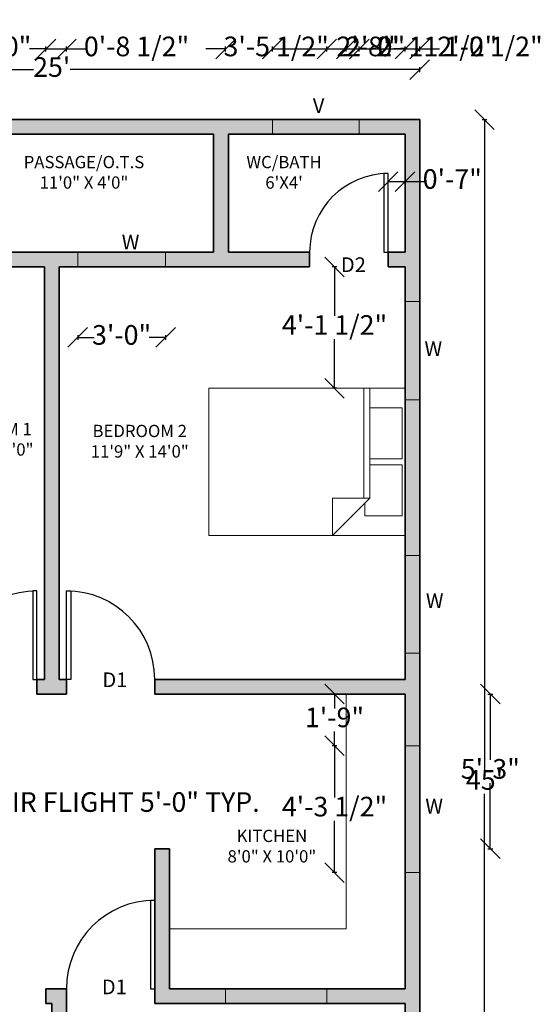
# Model space of a CAD drawing. Units: inches. Extents: x 2247 to 2713, y 588 to 1209.
# Tile 5 of 5: x 2501 to 2713, y 808 to 1209. Entities that reach past the tile are written whole.
import ezdxf

# ---------------------------------------------------------------- set-up
doc = ezdxf.new("R2010")
doc.units = ezdxf.units.IN
for name, color, linetype, lineweight in [('A-ANNO-DIMS', 2, 'Continuous', 18), ('A-ANNO-TEXT', 7, 'Continuous', 18), ('A-AREA-IDEN', 7, 'Continuous', 25), ('A-DOOR', 3, 'Continuous', 25), ('A-FLOR-FIXT', 9, 'Continuous', 18), ('A-FURN', 8, 'Continuous', 18), ('A-GLAZ', 4, 'Continuous', 18), ('A-GLAZ-PATT', 7, 'Continuous', 13), ('A-WALL', 7, 'Continuous', 35), ('A-WALL-PATT', 4, 'Continuous', 13)]:
    doc.layers.add(name, color=color, linetype=linetype, lineweight=lineweight)
doc.styles.get("Standard").update_dxf_attribs({"font": 'arial.ttf'})
doc.dimstyles.new('ISO-25', dxfattribs={"dimtxt": 8, "dimasz": 8, "dimexe": 1, "dimexo": 1, "dimtad": 0, "dimtih": 1, "dimtoh": 1, "dimlunit": 3, "dimtxsty": 'Standard', "dimblk": 'OBLIQUE', "dimcen": 2.5, "dimadec": 0, "dimazin": 0, "dimtfac": 1, "dimtmove": 0, "dimatfit": 3, "dimfxl": 1, "dimfxlon": 1, "dimarcsym": 0})

# ---------------------------------------------------------------- blocks, each defined once
blk = doc.blocks.new('*U4')
for p, q in [((0, 0), (0, -6)), ((-36, 0), (-36, -6))]:
    blk.add_line(p, q)
blk.add_lwpolyline([(0, 0), (0, 36), (-1.75, 36), (-1.75, 0)], close=True)
blk.add_arc((0, 0), 36, 90, 180)
blk = doc.blocks.new('*U6')
for p, q in [((0, 0), (0, -6)), ((-32, 0), (-32, -6))]:
    blk.add_line(p, q)
blk.add_lwpolyline([(0, 0), (0, 32), (-1.75, 32), (-1.75, 0)], close=True)
blk.add_arc((0, 0), 32, 90, 180)
blk = doc.blocks.new('*U5')
for p, q in [((0, 0), (0, -6)), ((36, 0), (36, -6))]:
    blk.add_line(p, q)
blk.add_lwpolyline([(0, 0), (0, 36), (1.75, 36), (1.75, 0)], close=True)
blk.add_arc((0, 0), 36, 0, 90)
blk = doc.blocks.new('Bed - Queen')
for p, q in [((0, -80.00003), (0, 0)), ((0, 0), (59.99999, 0)), ((59.99999, 0), (59.99999, -80.00003)), ((7.99999, -1.2), (28.79998, -1.2)), ((7.99999, -14.4), (7.99999, -1.2)), ((28.79998, -1.2), (28.79998, -14.4)), ((31.19999, -1.2), (51.99999, -1.2)), ((31.19999, -14.4), (31.19999, -1.2)), ((51.99999, -1.2), (51.99999, -16.4)), ((0, -14.4), (44.8, -14.4)), ((59.99999, -29.6), (44.8, -14.4)), ((44.8, -14.4), (44.8, -29.6)), ((44.8, -16.8), (0, -16.8)), ((51.99999, -16.4), (46.79936, -16.4)), ((44.8, -29.6), (59.99999, -29.6)), ((59.99999, -80.00003), (0, -80.00003))]:
    blk.add_line(p, q)
blk = doc.blocks.new('_Oblique')
at = {"color": 0, "linetype": 'ByBlock', "lineweight": -2}
blk.add_line((-0.5, -0.5), (0.5, 0.5), dxfattribs=at)
blk = doc.blocks.new('*D11')
at = {"layer": 'A-ANNO-DIMS', "color": 0, "lineweight": -2, "transparency": 16777216}
for p, q in [((2364.08, 1187.64), (2364.08, 1189.64)), ((2364.08, 1188.64), (2506.59, 1188.64)), ((2664.08, 1188.64), (2521.56, 1188.64)), ((2664.08, 1187.64), (2664.08, 1189.64))]:
    blk.add_line(p, q, dxfattribs=at)
at = {"layer": 'Defpoints', "color": 0, "transparency": 16777216}
for p in [(2664.08, 1188.64), (2364.08, 1168.28), (2664.08, 1168.28)]:
    blk.add_point(p, dxfattribs=at)
at = {"layer": 'A-ANNO-DIMS', "color": 0, "lineweight": -2, "transparency": 16777216, "xscale": 8, "yscale": 8, "zscale": 8, "rotation": 180}
blk.add_blockref('_Oblique', (2364.08, 1188.64), dxfattribs=at)
at = {"layer": 'A-ANNO-DIMS', "color": 0, "lineweight": -2, "transparency": 16777216, "xscale": 8, "yscale": 8, "zscale": 8}
blk.add_blockref('_Oblique', (2664.08, 1188.64), dxfattribs=at)
at = {"layer": 'A-ANNO-DIMS', "color": 0, "transparency": 16777216, "insert": (2514.08, 1188.64), "char_height": 8, "attachment_point": 5}
blk.add_mtext("25'", dxfattribs=at)
blk = doc.blocks.new('*D12')
at = {"layer": 'A-ANNO-DIMS', "color": 0, "lineweight": -2, "transparency": 16777216}
for p, q in [((2689.46, 1168.28), (2691.46, 1168.28)), ((2690.46, 1168.28), (2690.46, 902.97)), ((2690.46, 628.28), (2690.46, 893.59)), ((2689.46, 628.28), (2691.46, 628.28))]:
    blk.add_line(p, q, dxfattribs=at)
at = {"layer": 'Defpoints', "color": 0, "transparency": 16777216}
for p in [(2664.08, 1168.28), (2664.08, 628.28), (2690.46, 628.28)]:
    blk.add_point(p, dxfattribs=at)
at = {"layer": 'A-ANNO-DIMS', "color": 0, "lineweight": -2, "transparency": 16777216, "xscale": 8, "yscale": 8, "zscale": 8}
for p, rotation in [((2690.46, 1168.28), 90), ((2690.46, 628.28), 270)]:
    blk.add_blockref('_Oblique', p, dxfattribs=dict(at, rotation=rotation))
at = {"layer": 'A-ANNO-DIMS', "color": 0, "transparency": 16777216, "insert": (2690.46, 898.28), "char_height": 8, "attachment_point": 5}
blk.add_mtext("45'", dxfattribs=at)
blk = doc.blocks.new('*D17')
at = {"layer": 'A-ANNO-DIMS', "color": 0, "lineweight": -2, "transparency": 16777216}
for p, q in [((2406.08, 890.28), (2406.08, 888.28)), ((2466.08, 890.28), (2466.08, 888.28)), ((2406.08, 889.28), (2466.08, 889.28)), ((2466.08, 889.28), (2474.08, 889.28))]:
    blk.add_line(p, q, dxfattribs=at)
at = {"layer": 'Defpoints', "color": 0, "transparency": 16777216}
for p in [(2406.08, 898.28), (2466.08, 898.28), (2466.08, 889.28)]:
    blk.add_point(p, dxfattribs=at)
at = {"layer": 'A-ANNO-DIMS', "color": 0, "lineweight": -2, "transparency": 16777216, "xscale": 8, "yscale": 8, "zscale": 8, "rotation": 180}
blk.add_blockref('_Oblique', (2406.08, 889.28), dxfattribs=at)
at = {"layer": 'A-ANNO-DIMS', "color": 0, "lineweight": -2, "transparency": 16777216, "xscale": 8, "yscale": 8, "zscale": 8}
blk.add_blockref('_Oblique', (2466.08, 889.28), dxfattribs=at)
at = {"layer": 'A-ANNO-DIMS', "color": 0, "transparency": 16777216, "insert": (2538.49, 889.28), "char_height": 8, "attachment_point": 5}
blk.add_mtext('STAIR FLIGHT 5\'-0" TYP.', dxfattribs=at)
blk = doc.blocks.new('*D26')
at = {"layer": 'A-ANNO-DIMS', "color": 0, "lineweight": -2, "transparency": 16777216}
for p, q in [((2520.08, 600.53), (2520.08, 598.53)), ((2520.08, 599.53), (2526.82, 599.53)), ((2556.08, 599.53), (2549.33, 599.53)), ((2556.08, 600.53), (2556.08, 598.53))]:
    blk.add_line(p, q, dxfattribs=at)
at = {"layer": 'Defpoints', "color": 0, "transparency": 16777216}
for p in [(2520.08, 808.28), (2556.08, 808.28), (2556.08, 599.53)]:
    blk.add_point(p, dxfattribs=at)
at = {"layer": 'A-ANNO-DIMS', "color": 0, "lineweight": -2, "transparency": 16777216, "xscale": 8, "yscale": 8, "zscale": 8, "rotation": 180}
blk.add_blockref('_Oblique', (2520.08, 599.53), dxfattribs=at)
at = {"layer": 'A-ANNO-DIMS', "color": 0, "lineweight": -2, "transparency": 16777216, "xscale": 8, "yscale": 8, "zscale": 8}
blk.add_blockref('_Oblique', (2556.08, 599.53), dxfattribs=at)
at = {"layer": 'A-ANNO-DIMS', "color": 0, "transparency": 16777216, "insert": (2538.08, 599.53), "char_height": 8, "attachment_point": 5}
blk.add_mtext('3\'-0"', dxfattribs=at)
blk = doc.blocks.new('*D38')
at = {"layer": 'A-ANNO-DIMS', "color": 0, "lineweight": -2, "transparency": 16777216}
for p, q in [((2630.33, 913.24), (2628.33, 913.24)), ((2629.33, 913.24), (2629.33, 892.18)), ((2629.33, 861.58), (2629.33, 882.65)), ((2630.33, 861.58), (2628.33, 861.58))]:
    blk.add_line(p, q, dxfattribs=at)
at = {"layer": 'Defpoints', "color": 0, "transparency": 16777216}
for p in [(2629.33, 913.24), (2658.08, 913.24), (2658.08, 861.58)]:
    blk.add_point(p, dxfattribs=at)
at = {"layer": 'A-ANNO-DIMS', "color": 0, "lineweight": -2, "transparency": 16777216, "xscale": 8, "yscale": 8, "zscale": 8}
for p, rotation in [((2629.33, 913.24), 90), ((2629.33, 861.58), 270)]:
    blk.add_blockref('_Oblique', p, dxfattribs=dict(at, rotation=rotation))
at = {"layer": 'A-ANNO-DIMS', "color": 0, "transparency": 16777216, "insert": (2629.33, 887.41), "char_height": 8, "attachment_point": 5}
blk.add_mtext('4\'-3 1/2"', dxfattribs=at)
blk = doc.blocks.new('*D39')
at = {"layer": 'A-ANNO-DIMS', "color": 0, "lineweight": -2, "transparency": 16777216}
for p, q in [((2630.33, 934.28), (2628.33, 934.28)), ((2629.33, 934.28), (2629.33, 928.47)), ((2629.33, 913.24), (2629.33, 919.05)), ((2630.33, 913.24), (2628.33, 913.24))]:
    blk.add_line(p, q, dxfattribs=at)
at = {"layer": 'Defpoints', "color": 0, "transparency": 16777216}
for p in [(2629.33, 934.28), (2658.08, 934.28), (2658.08, 913.24)]:
    blk.add_point(p, dxfattribs=at)
at = {"layer": 'A-ANNO-DIMS', "color": 0, "lineweight": -2, "transparency": 16777216, "xscale": 8, "yscale": 8, "zscale": 8}
for p, rotation in [((2629.33, 934.28), 90), ((2629.33, 913.24), 270)]:
    blk.add_blockref('_Oblique', p, dxfattribs=dict(at, rotation=rotation))
at = {"layer": 'A-ANNO-DIMS', "color": 0, "transparency": 16777216, "insert": (2629.33, 923.76), "char_height": 8, "attachment_point": 5}
blk.add_mtext('1\'-9"', dxfattribs=at)
blk = doc.blocks.new('*D40')
at = {"layer": 'A-ANNO-DIMS', "color": 0, "lineweight": -2, "transparency": 16777216}
for p, q in [((2634.08, 1196.03), (2634.08, 1198.03)), ((2634.08, 1197.03), (2634.75, 1197.03)), ((2658.08, 1197.03), (2657.4, 1197.03)), ((2658.08, 1196.03), (2658.08, 1198.03))]:
    blk.add_line(p, q, dxfattribs=at)
at = {"layer": 'Defpoints', "color": 0, "transparency": 16777216}
for p in [(2658.08, 1197.03), (2634.08, 838.69), (2658.08, 814.28)]:
    blk.add_point(p, dxfattribs=at)
at = {"layer": 'A-ANNO-DIMS', "color": 0, "lineweight": -2, "transparency": 16777216, "xscale": 8, "yscale": 8, "zscale": 8, "rotation": 180}
blk.add_blockref('_Oblique', (2634.08, 1197.03), dxfattribs=at)
at = {"layer": 'A-ANNO-DIMS', "color": 0, "lineweight": -2, "transparency": 16777216, "xscale": 8, "yscale": 8, "zscale": 8}
blk.add_blockref('_Oblique', (2658.08, 1197.03), dxfattribs=at)
at = {"layer": 'A-ANNO-DIMS', "color": 0, "transparency": 16777216, "insert": (2646.08, 1197.03), "char_height": 8, "attachment_point": 5}
blk.add_mtext('2\'-0"', dxfattribs=at)
blk = doc.blocks.new('*D42')
at = {"layer": 'A-ANNO-DIMS', "color": 0, "lineweight": -2, "transparency": 16777216}
for p, q in [((2604.04, 1196.03), (2604.04, 1198.03)), ((2604.04, 1197.03), (2639.39, 1197.03)), ((2639.39, 1196.03), (2639.39, 1198.03)), ((2639.39, 1197.03), (2647.39, 1197.03))]:
    blk.add_line(p, q, dxfattribs=at)
at = {"layer": 'Defpoints', "color": 0, "transparency": 16777216}
for p in [(2639.39, 1197.03), (2604.04, 1168.28), (2639.39, 1168.28)]:
    blk.add_point(p, dxfattribs=at)
at = {"layer": 'A-ANNO-DIMS', "color": 0, "lineweight": -2, "transparency": 16777216, "xscale": 8, "yscale": 8, "zscale": 8, "rotation": 180}
blk.add_blockref('_Oblique', (2604.04, 1197.03), dxfattribs=at)
at = {"layer": 'A-ANNO-DIMS', "color": 0, "lineweight": -2, "transparency": 16777216, "xscale": 8, "yscale": 8, "zscale": 8}
blk.add_blockref('_Oblique', (2639.39, 1197.03), dxfattribs=at)
at = {"layer": 'A-ANNO-DIMS', "color": 0, "transparency": 16777216, "insert": (2671.15, 1197.03), "char_height": 8, "attachment_point": 5}
blk.add_mtext('2\'-11 1/2"', dxfattribs=at)
blk = doc.blocks.new('*D44')
at = {"layer": 'A-ANNO-DIMS', "color": 0, "lineweight": -2, "transparency": 16777216}
for p, q in [((2639.39, 1196.03), (2639.39, 1198.03)), ((2639.39, 1197.03), (2664.08, 1197.03)), ((2664.08, 1196.03), (2664.08, 1198.03)), ((2664.08, 1197.03), (2672.08, 1197.03))]:
    blk.add_line(p, q, dxfattribs=at)
at = {"layer": 'Defpoints', "color": 0, "transparency": 16777216}
for p in [(2664.08, 1197.03), (2639.39, 1168.28), (2664.08, 1168.28)]:
    blk.add_point(p, dxfattribs=at)
at = {"layer": 'A-ANNO-DIMS', "color": 0, "lineweight": -2, "transparency": 16777216, "xscale": 8, "yscale": 8, "zscale": 8, "rotation": 180}
blk.add_blockref('_Oblique', (2639.39, 1197.03), dxfattribs=at)
at = {"layer": 'A-ANNO-DIMS', "color": 0, "lineweight": -2, "transparency": 16777216, "xscale": 8, "yscale": 8, "zscale": 8}
blk.add_blockref('_Oblique', (2664.08, 1197.03), dxfattribs=at)
at = {"layer": 'A-ANNO-DIMS', "color": 0, "transparency": 16777216, "insert": (2692.72, 1197.03), "char_height": 8, "attachment_point": 5}
blk.add_mtext('2\'-0 1/2"', dxfattribs=at)
blk = doc.blocks.new('*D45')
at = {"layer": 'A-ANNO-DIMS', "color": 0, "lineweight": -2, "transparency": 16777216}
for p, q in [((2456.06, 600.53), (2456.06, 598.53)), ((2456.06, 599.53), (2487.37, 599.53)), ((2487.37, 600.53), (2487.37, 598.53)), ((2487.37, 599.53), (2495.37, 599.53))]:
    blk.add_line(p, q, dxfattribs=at)
at = {"layer": 'Defpoints', "color": 0, "transparency": 16777216}
for p in [(2456.06, 1108.28), (2487.37, 1108.28), (2487.37, 599.53)]:
    blk.add_point(p, dxfattribs=at)
at = {"layer": 'A-ANNO-DIMS', "color": 0, "lineweight": -2, "transparency": 16777216, "xscale": 8, "yscale": 8, "zscale": 8, "rotation": 180}
blk.add_blockref('_Oblique', (2456.06, 599.53), dxfattribs=at)
at = {"layer": 'A-ANNO-DIMS', "color": 0, "lineweight": -2, "transparency": 16777216, "xscale": 8, "yscale": 8, "zscale": 8}
blk.add_blockref('_Oblique', (2487.37, 599.53), dxfattribs=at)
at = {"layer": 'A-ANNO-DIMS', "color": 0, "transparency": 16777216, "insert": (2516.02, 599.53), "char_height": 8, "attachment_point": 5}
blk.add_mtext('2\'-7 1/2"', dxfattribs=at)
blk = doc.blocks.new('*D46')
at = {"layer": 'A-ANNO-DIMS', "color": 0, "lineweight": -2, "transparency": 16777216}
for p, q in [((2524.66, 1080.53), (2524.66, 1078.53)), ((2524.66, 1079.53), (2531.33, 1079.53)), ((2560.51, 1079.53), (2553.84, 1079.53)), ((2560.51, 1080.53), (2560.51, 1078.53))]:
    blk.add_line(p, q, dxfattribs=at)
at = {"layer": 'Defpoints', "color": 0, "transparency": 16777216}
for p in [(2524.66, 1108.28), (2560.51, 1108.28), (2524.66, 1079.53)]:
    blk.add_point(p, dxfattribs=at)
at = {"layer": 'A-ANNO-DIMS', "color": 0, "lineweight": -2, "transparency": 16777216, "xscale": 8, "yscale": 8, "zscale": 8, "rotation": 180}
blk.add_blockref('_Oblique', (2524.66, 1079.53), dxfattribs=at)
at = {"layer": 'A-ANNO-DIMS', "color": 0, "lineweight": -2, "transparency": 16777216, "xscale": 8, "yscale": 8, "zscale": 8}
blk.add_blockref('_Oblique', (2560.51, 1079.53), dxfattribs=at)
at = {"layer": 'A-ANNO-DIMS', "color": 0, "transparency": 16777216, "insert": (2542.58, 1079.53), "char_height": 8, "attachment_point": 5}
blk.add_mtext('3\'-0"', dxfattribs=at)
blk = doc.blocks.new('*D47')
at = {"layer": 'A-ANNO-DIMS', "color": 0, "lineweight": -2, "transparency": 16777216}
for p, q in [((2487.37, 600.53), (2487.37, 598.53)), ((2487.37, 599.53), (2524.66, 599.53)), ((2524.66, 600.53), (2524.66, 598.53)), ((2524.66, 599.53), (2532.66, 599.53))]:
    blk.add_line(p, q, dxfattribs=at)
at = {"layer": 'Defpoints', "color": 0, "transparency": 16777216}
for p in [(2487.37, 1108.28), (2524.66, 1108.28), (2524.66, 599.53)]:
    blk.add_point(p, dxfattribs=at)
at = {"layer": 'A-ANNO-DIMS', "color": 0, "lineweight": -2, "transparency": 16777216, "xscale": 8, "yscale": 8, "zscale": 8, "rotation": 180}
blk.add_blockref('_Oblique', (2487.37, 599.53), dxfattribs=at)
at = {"layer": 'A-ANNO-DIMS', "color": 0, "lineweight": -2, "transparency": 16777216, "xscale": 8, "yscale": 8, "zscale": 8}
blk.add_blockref('_Oblique', (2524.66, 599.53), dxfattribs=at)
at = {"layer": 'A-ANNO-DIMS', "color": 0, "transparency": 16777216, "insert": (2553.24, 599.53), "char_height": 8, "attachment_point": 5}
blk.add_mtext('3\'-1 1/2"', dxfattribs=at)
blk = doc.blocks.new('*D49')
at = {"layer": 'A-ANNO-DIMS', "color": 0, "lineweight": -2, "transparency": 16777216}
for p, q in [((2584.93, 1197.03), (2576.93, 1197.03)), ((2584.93, 1196.03), (2584.93, 1198.03)), ((2584.93, 1197.03), (2584.99, 1197.03)), ((2626.2, 1197.03), (2626.14, 1197.03)), ((2626.2, 1196.03), (2626.2, 1198.03)), ((2626.2, 1197.03), (2634.2, 1197.03))]:
    blk.add_line(p, q, dxfattribs=at)
at = {"layer": 'Defpoints', "color": 0, "transparency": 16777216}
for p in [(2626.2, 1197.03), (2584.93, 808.28), (2626.2, 808.28)]:
    blk.add_point(p, dxfattribs=at)
at = {"layer": 'A-ANNO-DIMS', "color": 0, "lineweight": -2, "transparency": 16777216, "xscale": 8, "yscale": 8, "zscale": 8}
blk.add_blockref('_Oblique', (2584.93, 1197.03), dxfattribs=at)
at = {"layer": 'A-ANNO-DIMS', "color": 0, "lineweight": -2, "transparency": 16777216, "xscale": 8, "yscale": 8, "zscale": 8, "rotation": 180}
blk.add_blockref('_Oblique', (2626.2, 1197.03), dxfattribs=at)
at = {"layer": 'A-ANNO-DIMS', "color": 0, "transparency": 16777216, "insert": (2605.57, 1197.03), "char_height": 8, "attachment_point": 5}
blk.add_mtext('3\'-5 1/2"', dxfattribs=at)
blk = doc.blocks.new('*D50')
at = {"layer": 'A-ANNO-DIMS', "color": 0, "lineweight": -2, "transparency": 16777216}
for p, q in [((2626.2, 1196.03), (2626.2, 1198.03)), ((2626.2, 1197.03), (2630.81, 1197.03)), ((2658.08, 1197.03), (2653.46, 1197.03)), ((2658.08, 1196.03), (2658.08, 1198.03))]:
    blk.add_line(p, q, dxfattribs=at)
at = {"layer": 'Defpoints', "color": 0, "transparency": 16777216}
for p in [(2658.08, 1197.03), (2626.2, 808.28), (2658.08, 808.28)]:
    blk.add_point(p, dxfattribs=at)
at = {"layer": 'A-ANNO-DIMS', "color": 0, "lineweight": -2, "transparency": 16777216, "xscale": 8, "yscale": 8, "zscale": 8, "rotation": 180}
blk.add_blockref('_Oblique', (2626.2, 1197.03), dxfattribs=at)
at = {"layer": 'A-ANNO-DIMS', "color": 0, "lineweight": -2, "transparency": 16777216, "xscale": 8, "yscale": 8, "zscale": 8}
blk.add_blockref('_Oblique', (2658.08, 1197.03), dxfattribs=at)
at = {"layer": 'A-ANNO-DIMS', "color": 0, "transparency": 16777216, "insert": (2642.14, 1197.03), "char_height": 8, "attachment_point": 5}
blk.add_mtext('2\'-8"', dxfattribs=at)
blk = doc.blocks.new('*D53')
at = {"layer": 'A-ANNO-DIMS', "color": 0, "lineweight": -2, "transparency": 16777216}
for p, q in [((2691.83, 934.28), (2693.83, 934.28)), ((2692.83, 934.28), (2692.83, 907.49)), ((2692.83, 871.28), (2692.83, 898.07)), ((2691.83, 871.28), (2693.83, 871.28))]:
    blk.add_line(p, q, dxfattribs=at)
at = {"layer": 'Defpoints', "color": 0, "transparency": 16777216}
for p in [(2556.08, 934.28), (2556.08, 871.28), (2692.83, 871.28)]:
    blk.add_point(p, dxfattribs=at)
at = {"layer": 'A-ANNO-DIMS', "color": 0, "lineweight": -2, "transparency": 16777216, "xscale": 8, "yscale": 8, "zscale": 8}
for p, rotation in [((2692.83, 934.28), 90), ((2692.83, 871.28), 270)]:
    blk.add_blockref('_Oblique', p, dxfattribs=dict(at, rotation=rotation))
at = {"layer": 'A-ANNO-DIMS', "color": 0, "transparency": 16777216, "insert": (2692.83, 902.78), "char_height": 8, "attachment_point": 5}
blk.add_mtext('5\'-3"', dxfattribs=at)
blk = doc.blocks.new('*D57')
at = {"layer": 'A-ANNO-DIMS', "color": 0, "lineweight": -2, "transparency": 16777216}
for p, q in [((2651.2, 1142.03), (2651.2, 1144.03)), ((2651.2, 1143.03), (2658.08, 1143.03)), ((2658.08, 1142.03), (2658.08, 1144.03)), ((2658.08, 1143.03), (2666.08, 1143.03))]:
    blk.add_line(p, q, dxfattribs=at)
at = {"layer": 'Defpoints', "color": 0, "transparency": 16777216}
for p in [(2658.08, 1143.03), (2651.2, 1114.28), (2658.08, 1114.28)]:
    blk.add_point(p, dxfattribs=at)
at = {"layer": 'A-ANNO-DIMS', "color": 0, "lineweight": -2, "transparency": 16777216, "xscale": 8, "yscale": 8, "zscale": 8, "rotation": 180}
blk.add_blockref('_Oblique', (2651.2, 1143.03), dxfattribs=at)
at = {"layer": 'A-ANNO-DIMS', "color": 0, "lineweight": -2, "transparency": 16777216, "xscale": 8, "yscale": 8, "zscale": 8}
blk.add_blockref('_Oblique', (2658.08, 1143.03), dxfattribs=at)
at = {"layer": 'A-ANNO-DIMS', "color": 0, "transparency": 16777216, "insert": (2677.33, 1143.03), "char_height": 8, "attachment_point": 5}
blk.add_mtext('0\'-7"', dxfattribs=at)
blk = doc.blocks.new('*D58')
at = {"layer": 'A-ANNO-DIMS', "color": 0, "lineweight": -2, "transparency": 16777216}
for p, q in [((2475.72, 1196.03), (2475.72, 1198.03)), ((2475.72, 1197.03), (2482.47, 1197.03)), ((2511.72, 1197.03), (2504.98, 1197.03)), ((2511.72, 1196.03), (2511.72, 1198.03))]:
    blk.add_line(p, q, dxfattribs=at)
at = {"layer": 'Defpoints', "color": 0, "transparency": 16777216}
for p in [(2511.72, 1197.03), (2475.72, 814.28), (2511.72, 814.28)]:
    blk.add_point(p, dxfattribs=at)
at = {"layer": 'A-ANNO-DIMS', "color": 0, "lineweight": -2, "transparency": 16777216, "xscale": 8, "yscale": 8, "zscale": 8, "rotation": 180}
blk.add_blockref('_Oblique', (2475.72, 1197.03), dxfattribs=at)
at = {"layer": 'A-ANNO-DIMS', "color": 0, "lineweight": -2, "transparency": 16777216, "xscale": 8, "yscale": 8, "zscale": 8}
blk.add_blockref('_Oblique', (2511.72, 1197.03), dxfattribs=at)
at = {"layer": 'A-ANNO-DIMS', "color": 0, "transparency": 16777216, "insert": (2493.72, 1197.03), "char_height": 8, "attachment_point": 5}
blk.add_mtext('3\'-0"', dxfattribs=at)
blk = doc.blocks.new('*D59')
at = {"layer": 'A-ANNO-DIMS', "color": 0, "lineweight": -2, "transparency": 16777216}
for p, q in [((2511.72, 1196.03), (2511.72, 1198.03)), ((2511.72, 1197.03), (2520.08, 1197.03)), ((2520.08, 1196.03), (2520.08, 1198.03)), ((2520.08, 1197.03), (2528.08, 1197.03))]:
    blk.add_line(p, q, dxfattribs=at)
at = {"layer": 'Defpoints', "color": 0, "transparency": 16777216}
for p in [(2520.08, 1197.03), (2511.72, 814.28), (2520.08, 814.28)]:
    blk.add_point(p, dxfattribs=at)
at = {"layer": 'A-ANNO-DIMS', "color": 0, "lineweight": -2, "transparency": 16777216, "xscale": 8, "yscale": 8, "zscale": 8, "rotation": 180}
blk.add_blockref('_Oblique', (2511.72, 1197.03), dxfattribs=at)
at = {"layer": 'A-ANNO-DIMS', "color": 0, "lineweight": -2, "transparency": 16777216, "xscale": 8, "yscale": 8, "zscale": 8}
blk.add_blockref('_Oblique', (2520.08, 1197.03), dxfattribs=at)
at = {"layer": 'A-ANNO-DIMS', "color": 0, "transparency": 16777216, "insert": (2548.65, 1197.03), "char_height": 8, "attachment_point": 5}
blk.add_mtext('0\'-8 1/2"', dxfattribs=at)
blk = doc.blocks.new('*D61')
at = {"layer": 'A-ANNO-DIMS', "color": 0, "lineweight": -2, "transparency": 16777216}
for p, q in [((2630.33, 1108.28), (2628.33, 1108.28)), ((2629.33, 1108.28), (2629.33, 1088.33)), ((2629.33, 1058.86), (2629.33, 1078.81)), ((2630.33, 1058.86), (2628.33, 1058.86))]:
    blk.add_line(p, q, dxfattribs=at)
at = {"layer": 'Defpoints', "color": 0, "transparency": 16777216}
for p in [(2629.33, 1108.28), (2658.08, 1108.28), (2658.08, 1058.86)]:
    blk.add_point(p, dxfattribs=at)
at = {"layer": 'A-ANNO-DIMS', "color": 0, "lineweight": -2, "transparency": 16777216, "xscale": 8, "yscale": 8, "zscale": 8}
for p, rotation in [((2629.33, 1108.28), 90), ((2629.33, 1058.86), 270)]:
    blk.add_blockref('_Oblique', p, dxfattribs=dict(at, rotation=rotation))
at = {"layer": 'A-ANNO-DIMS', "color": 0, "transparency": 16777216, "insert": (2629.33, 1083.57), "char_height": 8, "attachment_point": 5}
blk.add_mtext('4\'-1 1/2"', dxfattribs=at)

msp = doc.modelspace()

# ---------------------------------------------------------------- hatches: boundary and pattern name
at = {"layer": 'A-GLAZ-PATT'}
h = msp.add_hatch(color=256, dxfattribs=at)
h.dxf.hatch_style = 1
h.paths.add_polyline_path([(2423.716, 1168.28), (2380.833, 1168.28), (2380.833, 1162.28), (2423.716, 1162.28)])
h.paths.add_polyline_path([(2487.371, 1114.28), (2456.056, 1114.28), (2456.056, 1108.28), (2487.371, 1108.28)])
h.paths.add_polyline_path([(2560.507, 1114.28), (2524.66, 1114.28), (2524.66, 1108.28), (2560.507, 1108.28)])
h.paths.add_polyline_path([(2639.393, 1168.28), (2604.041, 1168.28), (2604.041, 1162.28), (2639.393, 1162.28)])
h.paths.add_polyline_path([(2370.076, 1094.128), (2364.076, 1094.128), (2364.076, 1054.172), (2370.076, 1054.172), (2370.076, 1068.35)])
h.paths.add_polyline_path([(2370.076, 990.686), (2364.076, 990.686), (2364.076, 950.99), (2370.076, 950.99)])
h.paths.add_polyline_path([(2664.076, 1094.128), (2658.076, 1094.128), (2658.076, 1054.172), (2664.076, 1054.172)])
h.paths.add_polyline_path([(2664.076, 990.686), (2658.076, 990.686), (2658.076, 950.99), (2664.076, 950.99)])
h.paths.add_polyline_path([(2664.076, 913.24), (2658.076, 913.24), (2658.076, 861.585), (2664.076, 861.585)])
h.paths.add_polyline_path([(2626.201, 814.28), (2584.934, 814.28), (2584.934, 808.28), (2626.201, 808.28)])
h.paths.add_polyline_path([(2370.076, 902.687), (2364.076, 902.687), (2364.076, 846.663), (2370.076, 846.663)])
h.paths.add_polyline_path([(2370.076, 776.746), (2364.076, 776.746), (2364.076, 709.673), (2370.076, 709.673)])
h.paths.add_polyline_path([(2457.582, 679.28), (2410.479, 679.28), (2410.479, 673.28), (2457.582, 673.28)])
at = {"layer": 'A-WALL-PATT'}
h = msp.add_hatch(color=256, dxfattribs=at)
h.dxf.hatch_style = 1
h.paths.add_polyline_path([(2604.041, 1168.28), (2423.716, 1168.28), (2423.716, 1162.28), (2442.076, 1162.28), (2442.076, 1114.28), (2439.021, 1114.28), (2439.021, 1108.28), (2456.056, 1108.28), (2456.056, 1114.28), (2448.076, 1114.28), (2448.076, 1162.28), (2580.076, 1162.28), (2580.076, 1114.28), (2560.507, 1114.28), (2560.507, 1108.28), (2619.195, 1108.28), (2619.195, 1114.28), (2586.076, 1114.28), (2586.076, 1162.28), (2604.041, 1162.28)])
h.paths.add_polyline_path([(2380.833, 1168.28), (2364.076, 1168.28), (2364.076, 1094.128), (2370.076, 1094.128), (2370.076, 1108.28), (2407.021, 1108.28), (2407.021, 1114.28), (2370.076, 1114.28), (2370.076, 1162.28), (2380.833, 1162.28)])
h.paths.add_polyline_path([(2664.076, 1168.28), (2639.393, 1168.28), (2639.393, 1162.28), (2658.076, 1162.28), (2658.076, 1114.28), (2651.195, 1114.28), (2651.195, 1108.28), (2658.076, 1108.28), (2658.076, 1094.128), (2664.076, 1094.128)])
h.paths.add_polyline_path([(2524.66, 1114.28), (2487.371, 1114.28), (2487.371, 1108.28), (2511.076, 1108.28), (2511.076, 940.28), (2508.076, 940.28), (2508.076, 934.28), (2520.076, 934.28), (2520.076, 940.28), (2517.076, 940.28), (2517.076, 1108.28), (2524.66, 1108.28)])
h.paths.add_polyline_path([(2370.076, 1054.172), (2364.076, 1054.172), (2364.076, 990.686), (2370.076, 990.686)])
h.paths.add_polyline_path([(2370.076, 934.28), (2472.076, 934.28), (2472.076, 940.28), (2370.076, 940.28), (2370.076, 950.99), (2364.076, 950.99), (2364.076, 902.687), (2370.076, 902.687)])
h.paths.add_polyline_path([(2664.076, 950.99), (2658.076, 950.99), (2658.076, 940.28), (2556.076, 940.28), (2556.076, 934.28), (2658.076, 934.28), (2658.076, 913.24), (2664.076, 913.24)])
h.paths.add_polyline_path([(2664.076, 1054.172), (2658.076, 1054.172), (2658.076, 990.686), (2664.076, 990.686)])
h.paths.add_polyline_path([(2664.076, 861.585), (2658.076, 861.585), (2658.076, 814.28), (2626.201, 814.28), (2626.201, 808.28), (2658.076, 808.28), (2658.076, 628.28), (2664.076, 628.28)])
h.paths.add_polyline_path([(2562.076, 871.28), (2556.076, 871.28), (2556.076, 808.28), (2584.934, 808.28), (2584.934, 814.28), (2562.076, 814.28)])
h.paths.add_polyline_path([(2475.722, 808.28), (2370.076, 808.28), (2370.076, 776.746), (2364.076, 776.746), (2364.076, 846.663), (2370.076, 846.663), (2370.076, 814.28), (2475.722, 814.28)])
h.paths.add_polyline_path([(2370.076, 709.673), (2364.076, 709.673), (2364.076, 628.28), (2520.076, 628.28), (2520.076, 634.28), (2370.076, 634.28)])
h.paths.add_polyline_path([(2410.479, 679.28), (2370.076, 679.28), (2370.076, 673.28), (2410.479, 673.28)], flags=17)
h.paths.add_polyline_path([(2520.076, 679.28), (2514.076, 679.28), (2474.076, 679.28), (2457.582, 679.28), (2457.582, 673.28), (2520.076, 673.28)], flags=17)
h.paths.add_polyline_path([(2520.076, 814.28), (2511.722, 814.28), (2511.722, 808.28), (2514.076, 808.28), (2514.076, 719.28), (2520.076, 719.28)])

# ---------------------------------------------------------------- linework, layer by layer
at = {"layer": 'A-FLOR-FIXT'}
for p, q in [((2634.076, 838.687), (2634.076, 934.28)), ((2562.076, 838.687), (2634.076, 838.687))]:
    msp.add_line(p, q, dxfattribs=at)
at = {"layer": 'A-GLAZ'}
for p, q in [((2604.041, 1162.28), (2604.041, 1168.28)), ((2639.393, 1162.28), (2639.393, 1168.28)), ((2524.66, 1114.28), (2524.66, 1108.28)), ((2560.507, 1114.28), (2560.507, 1108.28)), ((2664.076, 1094.128), (2658.076, 1094.128)), ((2658.076, 1054.172), (2664.076, 1054.172)), ((2658.076, 990.686), (2664.076, 990.686)), ((2664.076, 950.99), (2658.076, 950.99)), ((2658.076, 913.24), (2664.076, 913.24)), ((2658.076, 861.585), (2664.076, 861.585)), ((2584.934, 814.28), (2584.934, 808.28)), ((2626.201, 814.28), (2626.201, 808.28))]:
    msp.add_line(p, q, dxfattribs=at)
at = {"layer": 'A-WALL'}
for p, q in [((2664.076, 1168.28), (2364.076, 1168.28)), ((2664.076, 628.28), (2664.076, 1168.28)), ((2580.076, 1162.28), (2448.076, 1162.28)), ((2580.076, 1162.28), (2580.076, 1114.28)), ((2658.076, 1162.28), (2586.076, 1162.28)), ((2586.076, 1162.28), (2586.076, 1114.28)), ((2658.076, 1114.28), (2658.076, 1162.28)), ((2580.076, 1114.28), (2448.076, 1114.28)), ((2619.195, 1114.28), (2586.076, 1114.28)), ((2619.195, 1114.28), (2619.195, 1108.28)), ((2658.076, 1114.28), (2651.195, 1114.28)), ((2651.195, 1114.28), (2651.195, 1108.28)), ((2511.076, 1108.28), (2439.021, 1108.28)), ((2511.076, 1108.28), (2511.076, 940.28)), ((2517.076, 940.28), (2517.076, 1108.28)), ((2619.195, 1108.28), (2517.076, 1108.28)), ((2658.076, 1108.28), (2651.195, 1108.28)), ((2658.076, 940.28), (2658.076, 1108.28)), ((2511.076, 940.28), (2508.076, 940.28)), ((2508.076, 940.28), (2508.076, 934.28)), ((2520.076, 940.28), (2517.076, 940.28)), ((2520.076, 934.28), (2520.076, 940.28)), ((2658.076, 940.28), (2556.076, 940.28)), ((2556.076, 934.28), (2556.076, 940.28)), ((2520.076, 934.28), (2508.076, 934.28)), ((2658.076, 934.28), (2556.076, 934.28)), ((2658.076, 814.28), (2658.076, 934.28)), ((2556.076, 808.28), (2556.076, 871.28)), ((2562.076, 871.28), (2556.076, 871.28)), ((2562.076, 814.28), (2562.076, 871.28)), ((2520.076, 814.28), (2511.722, 814.28)), ((2511.722, 808.28), (2511.722, 814.28)), ((2520.076, 719.28), (2520.076, 814.28)), ((2658.076, 814.28), (2562.076, 814.28)), ((2514.076, 808.28), (2511.722, 808.28)), ((2514.076, 719.28), (2514.076, 808.28)), ((2658.076, 808.28), (2556.076, 808.28)), ((2658.076, 628.28), (2658.076, 808.28))]:
    msp.add_line(p, q, dxfattribs=at)

# ---------------------------------------------------------------- block references
at = {"layer": 'A-DOOR'}
for name, p in [('*U6', (2651.195, 1114.28)), ('*U4', (2508.076, 940.28)), ('*U5', (2520.076, 940.28)), ('*U4', (2556.076, 814.28))]:
    msp.add_blockref(name, p, dxfattribs=at)
at = {"layer": 'A-FURN', "rotation": 270}
msp.add_blockref('Bed - Queen', (2658.076, 1058.864), dxfattribs=at)

# ---------------------------------------------------------------- texts
at = {"layer": 'A-ANNO-TEXT', "char_height": 6, "attachment_point": 1}
for s, insert in [('\\pxqc;V', (2616.902, 1176.944)), ('\\pxqc;W', (2540.256, 1121.364)), ('\\pxqc;D2', (2631.073, 1112.165)), ('\\pxqc;W', (2663.64, 1077.955)), ('\\pxqc;W', (2664.203, 975.329)), ('\\pxqc;D1', (2533.882, 943.115)), ('\\pxqc;W', (2663.987, 891.647)), ('\\pxqc;D1', (2533.648, 818.007))]:
    msp.add_mtext_dynamic_manual_height_columns(s, width=11.90357, gutter_width=12.5, heights=[0], dxfattribs=dict(at, insert=insert))
at = {"layer": 'A-AREA-IDEN', "char_height": 5, "attachment_point": 1}
for s, width, insert in [('\\pxqc;PASSAGE/O.T.S\\P11\'0" X 4\'0"', 77.01258, (2488.725, 1153.469)), ("\\pxqc;WC/BATH\\P6'X4'", 33.16994, (2592.182, 1153.469)), ('\\pxqc;BEDROOM 1\\P11\'9" X 14\'0"', 45.05776, (2464.156, 1044.727)), ('\\pxqc;BEDROOM 2\\P11\'9" X 14\'0"', 47.44598, (2526.232, 1043.952)), ('\\pxqc;KITCHEN\\P8\'0" X 10\'0"', 42.14785, (2582.743, 879.028))]:
    msp.add_mtext_dynamic_manual_height_columns(s, width=width, gutter_width=12.5, heights=[0], dxfattribs=dict(at, insert=insert))

# ---------------------------------------------------------------- dimensions: what is measured, and where the dimension line sits
at = {"layer": 'A-ANNO-DIMS'}
for base, p1, p2, override, picture, middle in [((2520.076, 1197.03), (2511.722, 814.28), (2520.076, 814.28), {"dimdec": 1, "dimlfac": 1, "dimrnd": 0, "dimzin": 1, "dimdsep": 46, "dimlunit": 4, "dimfrac": 2}, '*D59', (2548.655, 1197.03)), ((2626.201, 1197.03), (2584.934, 808.28), (2626.201, 808.28), {"dimdec": 1, "dimlfac": 1, "dimrnd": 0, "dimzin": 1, "dimdsep": 46, "dimlunit": 4, "dimfrac": 2}, '*D49', (2605.568, 1197.03)), ((2639.393, 1197.03), (2604.041, 1168.28), (2639.393, 1168.28), {"dimdec": 1, "dimlfac": 1, "dimrnd": 0, "dimzin": 1, "dimdsep": 46, "dimlunit": 4, "dimfrac": 2}, '*D42', (2671.147, 1197.03)), ((2664.076, 1197.03), (2639.393, 1168.28), (2664.076, 1168.28), {"dimdec": 1, "dimlfac": 1, "dimrnd": 0, "dimzin": 1, "dimdsep": 46, "dimlunit": 4, "dimfrac": 2}, '*D44', (2692.723, 1197.03)), ((2511.722, 1197.03), (2475.722, 814.28), (2511.722, 814.28), {"dimdec": 1, "dimlfac": 1, "dimrnd": 0, "dimzin": 1, "dimdsep": 46, "dimlunit": 4, "dimfrac": 2}, '*D58', (2493.722, 1197.03)), ((2658.076, 1197.03), (2626.201, 808.28), (2658.076, 808.28), {"dimdec": 1, "dimlfac": 1, "dimrnd": 0, "dimzin": 1, "dimdsep": 46, "dimlunit": 4, "dimfrac": 2}, '*D50', (2642.139, 1197.03)), ((2658.076, 1197.03), (2634.076, 838.687), (2658.076, 814.28), {"dimdec": 1, "dimlfac": 1, "dimrnd": 0, "dimzin": 1, "dimdsep": 46, "dimlunit": 4, "dimfrac": 2}, '*D40', (2646.076, 1197.03)), ((2664.076, 1188.641), (2364.076, 1168.28), (2664.076, 1168.28), {"dimclrd": 0, "dimclre": 0, "dimclrt": 0}, '*D11', (2514.076, 1188.641)), ((2658.076, 1143.03), (2651.195, 1114.28), (2658.076, 1114.28), {"dimdec": 1, "dimlfac": 1, "dimrnd": 0, "dimzin": 1, "dimdsep": 46, "dimlunit": 4, "dimfrac": 2}, '*D57', (2677.334, 1143.03)), ((2487.371, 599.53), (2456.056, 1108.28), (2487.371, 1108.28), {"dimdec": 1, "dimlfac": 1, "dimrnd": 0, "dimzin": 1, "dimdsep": 46, "dimlunit": 4, "dimfrac": 2}, '*D45', (2516.018, 599.53)), ((2524.66, 599.53), (2487.371, 1108.28), (2524.66, 1108.28), {"dimdec": 1, "dimlfac": 1, "dimrnd": 0, "dimzin": 1, "dimdsep": 46, "dimlunit": 4, "dimfrac": 2}, '*D47', (2553.236, 599.53)), ((2556.076, 599.53), (2520.076, 808.28), (2556.076, 808.28), {"dimdec": 1, "dimlfac": 1, "dimrnd": 0, "dimzin": 1, "dimdsep": 46, "dimlunit": 4, "dimfrac": 2}, '*D26', (2538.076, 599.53))]:
    dim = msp.add_linear_dim(base=base, p1=p1, p2=p2, dimstyle='ISO-25', override=override, dxfattribs=at)
    dim.commit()
    dim.dimension.update_dxf_attribs({"geometry": picture, "text_midpoint": middle})
for base, p1, p2, angle, override, picture, middle in [((2690.46, 628.28), (2664.076, 1168.28), (2664.076, 628.28), 90, {"dimclrd": 0, "dimclre": 0, "dimclrt": 0}, '*D12', (2690.46, 898.28)), ((2629.326, 1108.28), (2658.076, 1058.864), (2658.076, 1108.28), 90, {"dimdec": 1, "dimlfac": 1, "dimrnd": 0, "dimzin": 1, "dimdsep": 46, "dimlunit": 4, "dimfrac": 2}, '*D61', (2629.326, 1083.572)), ((2524.66, 1079.53), (2560.507, 1108.28), (2524.66, 1108.28), 180, {"dimdec": 1, "dimlfac": 1, "dimrnd": 0, "dimzin": 1, "dimdsep": 46, "dimlunit": 4, "dimfrac": 2}, '*D46', (2542.584, 1079.53)), ((2692.826, 871.28), (2556.076, 934.28), (2556.076, 871.28), 90, {"dimdec": 1, "dimlfac": 1, "dimrnd": 0, "dimzin": 1, "dimdsep": 46, "dimlunit": 4, "dimfrac": 2}, '*D53', (2692.826, 902.78)), ((2629.326, 934.28), (2658.076, 913.24), (2658.076, 934.28), 90, {"dimdec": 1, "dimlfac": 1, "dimrnd": 0, "dimzin": 1, "dimdsep": 46, "dimlunit": 4, "dimfrac": 2}, '*D39', (2629.326, 923.76)), ((2629.326, 913.24), (2658.076, 861.585), (2658.076, 913.24), 90, {"dimdec": 1, "dimlfac": 1, "dimrnd": 0, "dimzin": 1, "dimdsep": 46, "dimlunit": 4, "dimfrac": 2}, '*D38', (2629.326, 887.412))]:
    dim = msp.add_linear_dim(base=base, p1=p1, p2=p2, angle=angle, dimstyle='ISO-25', override=override, dxfattribs=at)
    dim.commit()
    dim.dimension.update_dxf_attribs({"geometry": picture, "text_midpoint": middle})
dim = msp.add_linear_dim(base=(2466.076, 889.28), p1=(2406.076, 898.28), p2=(2466.076, 898.28), text='STAIR FLIGHT <> TYP.', dimstyle='ISO-25', override={"dimdec": 1, "dimlfac": 1, "dimrnd": 0, "dimzin": 1, "dimdsep": 46, "dimlunit": 4, "dimfrac": 2}, dxfattribs=at)
dim.commit()
dim.dimension.update_dxf_attribs({"geometry": '*D17', "text_midpoint": (2538.494, 889.28)})

doc.saveas('drawing.dxf')
